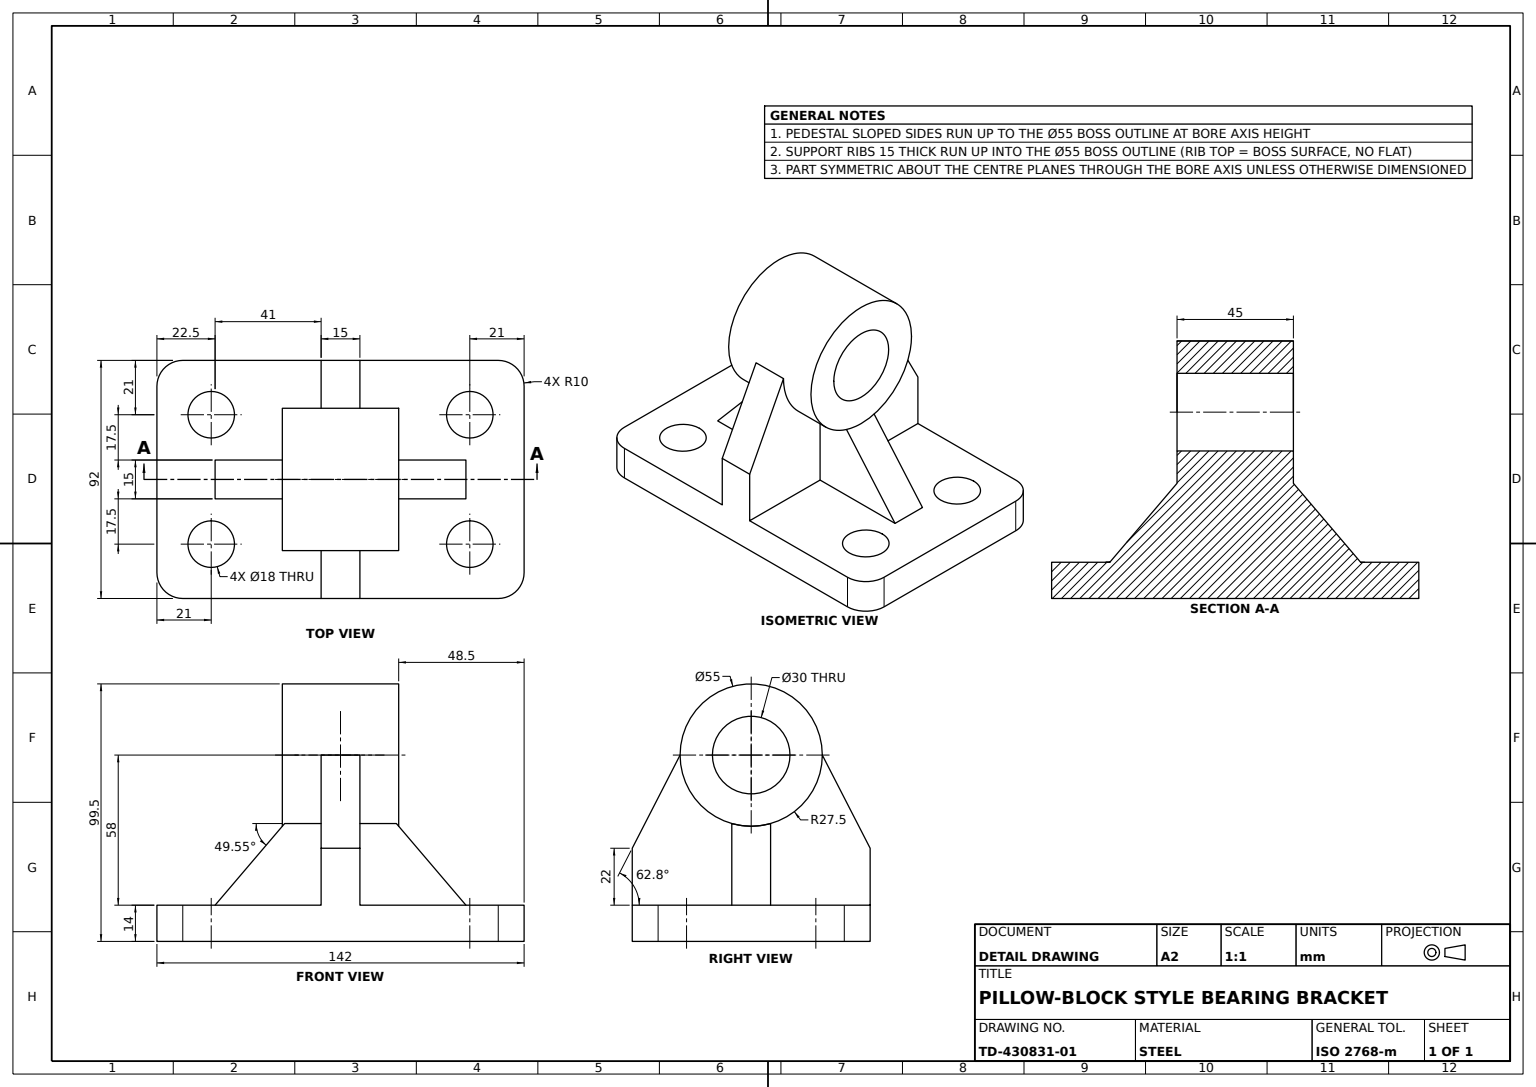
from build123d import *

# Parameters (mm, degrees)
BASE_PLATE_SKETCH_W         = 142
BASE_PLATE_SKETCH_H         = 92
BASE_PLATE_142X92X14_DEPTH  = 14
BASE_CORNER_FILLETS_R10_R   = 10
BEARING_PEDESTAL_DEPTH      = 7.5
BEARING_BOSS_SKETCH_R       = 27.5
BEARING_BOSS_55_DEPTH       = 22.5
BORE_SKETCH_R               = 15
BORE_30_DEPTH               = 145.078103819
SUPPORT_RIB_1_REACH         = 132.603
SUPPORT_RIB_1_SKETCH_WALL_W = 303.284863468
SUPPORT_RIB_1_SKETCH_WALL_H = 15
SUPPORT_RIB_2_REACH         = 132.603
SUPPORT_RIB_2_SKETCH_WALL_W = 303.284863468
SUPPORT_RIB_2_SKETCH_WALL_H = 15
MOUNTING_HOLES_SKETCH_R     = 9
MOUNTING_HOLES_4X_18_DEPTH  = 41


with BuildPart() as part:
    # Base Plate Sketch → Base Plate 142x92x14 (new body)
    with BuildSketch(Plane(origin=(0, 0, 0), x_dir=(1, 0, 0), z_dir=(0, 1, 0))):
        Rectangle(BASE_PLATE_SKETCH_W, BASE_PLATE_SKETCH_H)
    extrude(amount=BASE_PLATE_142X92X14_DEPTH)

    # Base Corner Fillets R10
    base_corner_fillets_r10_edges = [part.edges().sort_by_distance(p)[0] for p in [
        (71, 7, 46),
        (-71, 7, 46),
        (-71, 7, -46),
        (71, 7, -46),
    ]]
    fillet(base_corner_fillets_r10_edges, radius=BASE_CORNER_FILLETS_R10_R)

    # Pedestal Sketch → Bearing Pedestal (add, symmetric)
    with BuildSketch(Plane(origin=(0, 0, 0), x_dir=(0, 0, -1), z_dir=(1, 0, 0))):
        Polygon((46, 14), (46, 36), (27.50046584, 72), (-27.49953416, 72), (-46, 36), (-46, 14), align=None)
    extrude(amount=BEARING_PEDESTAL_DEPTH, both=True)

    # Bearing Boss Sketch → Bearing Boss Ø55 (add, symmetric)
    with BuildSketch(Plane(origin=(0, 0, 0), x_dir=(0, 0, -1), z_dir=(1, 0, 0))):
        with Locations((0.00046584, 72)):
            Circle(BEARING_BOSS_SKETCH_R)
    extrude(amount=BEARING_BOSS_55_DEPTH, both=True)

    # Bore Sketch → Bore Ø30 (cut, through all)
    with BuildSketch(Plane(origin=(22.5, 0, 0), x_dir=(0, 0, -1), z_dir=(1, 0, 0))):
        with Locations((0.00046584, 72)):
            Circle(BORE_SKETCH_R)
    extrude(amount=-BORE_30_DEPTH, mode=Mode.SUBTRACT)

    # Support Rib 1 Sketch wall → Support Rib 1 (add, up to next)
    with BuildSketch(Plane(origin=(35.5, 29.25, 0), x_dir=(0.648734176014, -0.761015091093, 0), z_dir=(0.761015091093, 0.648734176014, 0)), mode=Mode.PRIVATE) as support_rib_1_sk1:
        Rectangle(SUPPORT_RIB_1_SKETCH_WALL_W, SUPPORT_RIB_1_SKETCH_WALL_H)
    support_rib_1_tool1 = extrude(support_rib_1_sk1.sketch, amount=-SUPPORT_RIB_1_REACH, mode=Mode.PRIVATE) - part.part
    add(support_rib_1_tool1.solids().sort_by_distance((35.5, 29.25, 0))[0])

    # Support Rib 2 Sketch wall → Support Rib 2 (add, up to next)
    with BuildSketch(Plane(origin=(-35.5, 29.25, 0), x_dir=(-0.648734176014, -0.761015091093, 0), z_dir=(0.761015091093, -0.648734176014, 0)), mode=Mode.PRIVATE) as support_rib_2_sk1:
        Rectangle(SUPPORT_RIB_2_SKETCH_WALL_W, SUPPORT_RIB_2_SKETCH_WALL_H)
    support_rib_2_tool1 = extrude(support_rib_2_sk1.sketch, amount=SUPPORT_RIB_2_REACH, mode=Mode.PRIVATE) - part.part
    add(support_rib_2_tool1.solids().sort_by_distance((-35.5, 29.25, 0))[0])

    # Mounting Holes Sketch → Mounting Holes 4xØ18 (cut)
    with BuildSketch(Plane(origin=(0, 14, 0), x_dir=(1, 0, 0), z_dir=(0, 1, 0))):
        with Locations(Location((-50, 25, 0), (0, 0, 270))):
            Circle(MOUNTING_HOLES_SKETCH_R)
        with Locations(Location((50, 25, 0), (0, 0, 270))):
            Circle(MOUNTING_HOLES_SKETCH_R)
        with Locations(Location((50, -25, 0), (0, 0, 270))):
            Circle(MOUNTING_HOLES_SKETCH_R)
        with Locations(Location((-50, -25, 0), (0, 0, 270))):
            Circle(MOUNTING_HOLES_SKETCH_R)
    extrude(amount=-MOUNTING_HOLES_4X_18_DEPTH, mode=Mode.SUBTRACT)


solid = part.part
